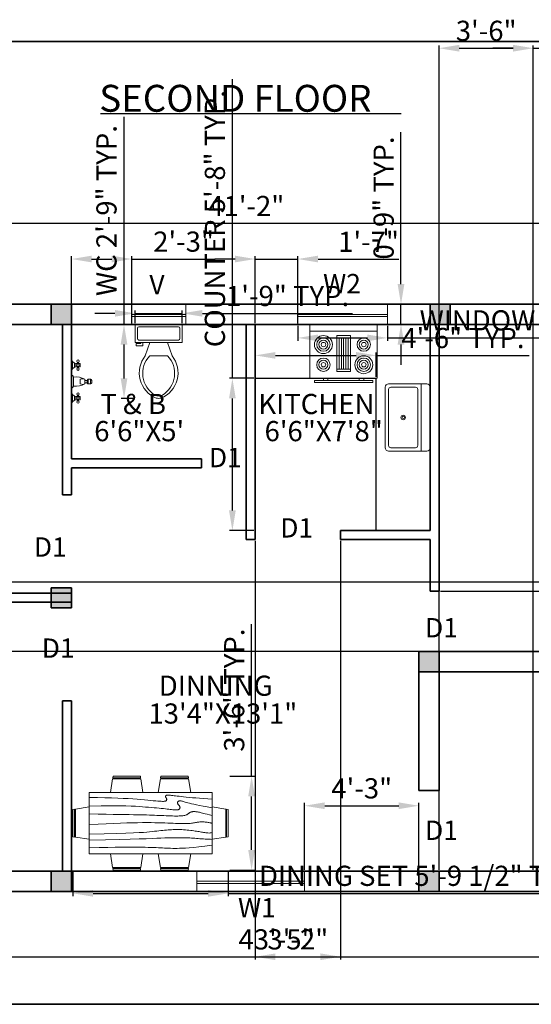
# Model space of a CAD drawing. Units: inches. Extents: x -281 to 2337, y 1647 to 2113.
# Tile 2 of 6: x 1230 to 1459, y 1674 to 2113. Entities that reach past the tile are written whole.
import ezdxf

# ---------------------------------------------------------------- set-up
doc = ezdxf.new("R2010")
doc.units = ezdxf.units.IN
for name, color, linetype, lineweight in [('A-ANNO-DIMS', 242, 'Continuous', 18), ('A-ANNO-IDEN', 11, 'Continuous', 18), ('A-ANNO-TEXT', 7, 'Continuous', 25), ('A-ANNO-TTLB', 7, 'Continuous', 35), ('A-AREA-IDEN', 7, 'Continuous', 18), ('A-COLS', 1, 'Continuous', 35), ('A-EQPM', 8, 'Continuous', 18), ('A-FLOR-CASE', 8, 'Continuous', 25), ('A-FLOR-FIXT', 8, 'Continuous', 18), ('A-FURN', 8, 'Continuous', 18), ('A-GLAZ', 3, 'Continuous', 18), ('A-WALL', 7, 'Continuous', 35)]:
    doc.layers.add(name, color=color, linetype=linetype, lineweight=lineweight)
doc.styles.get("Standard").update_dxf_attribs({"font": 'arial.ttf'})
doc.dimstyles.new('ISO-25', dxfattribs={"dimtxt": 9, "dimasz": 9, "dimexe": 1.25, "dimexo": 0.625, "dimgap": 2, "dimtad": 1, "dimdec": 1, "dimlunit": 4, "dimtxsty": 'Standard', "dimcen": 2.5, "dimadec": 0, "dimazin": 0, "dimtfac": 1, "dimtdec": 1, "dimtmove": 0, "dimatfit": 3, "dimfxl": 1, "dimarcsym": 0})

# ---------------------------------------------------------------- blocks, each defined once
blk = doc.blocks.new('Dining Set - 36 x 72 in.')
for p, q in [((-22.2343, 26.00059), (-23.4847, 17.99762)), ((-22.2304, 26), (-5.7608, 26)), ((-22, 27.5), (-22.1562, 26.50042)), ((-5.8416, 26.5), (-22.1534, 26.5)), ((-22, 27.5), (-6, 27.5)), ((-5.8437, 26.49966), (-6, 27.5)), ((-4.5152, 17.99762), (-5.7655, 25.99926)), ((5.7657, 26.00059), (4.5153, 17.99762)), ((5.7696, 26), (22.2392, 26)), ((6, 27.5), (5.8438, 26.50042)), ((22.1584, 26.5), (5.8466, 26.5)), ((6, 27.5), (22, 27.5)), ((22.1563, 26.49966), (22, 27.5)), ((23.4848, 17.99762), (22.2345, 25.99926)), ((36, 18), (-36, 18)), ((-36, 18), (-36, -18)), ((36, -18), (36, 18)), ((-45.5, 8), (-44.5004, 8.15617)), ((-45.5, 8), (-45.5, -8)), ((-44.5, -8.15843), (-44.5, 8.15338)), ((-44.0006, 8.23428), (-35.9976, 9.48474)), ((-44, 8.23041), (-44, -8.23915)), ((44.0006, 8.23428), (35.9976, 9.48474)), ((44, 8.23041), (44, -8.23915)), ((44.5, -8.15843), (44.5, 8.15338)), ((45.5, 8), (44.5005, 8.15617)), ((45.5, 8), (45.5, -8)), ((-44.4997, -8.15631), (-45.5, -8)), ((-35.9976, -9.48476), (-43.9993, -8.2345)), ((35.9976, -9.48476), (43.9993, -8.2345)), ((44.4997, -8.15631), (45.5, -8)), ((-36, -18), (36, -18)), ((-22.2343, -26.0006), (-23.4847, -17.99762)), ((-4.5152, -17.99762), (-5.7655, -25.99928)), ((5.7657, -26.0006), (4.5153, -17.99762)), ((23.4848, -17.99762), (22.2345, -25.99928)), ((-22.2304, -26), (-5.7608, -26)), ((-22, -27.5), (-22.1562, -26.50044)), ((-5.8416, -26.5), (-22.1534, -26.5)), ((-22, -27.5), (-6, -27.5)), ((-5.8437, -26.49967), (-6, -27.5)), ((5.7696, -26), (22.2392, -26)), ((6, -27.5), (5.8438, -26.50044)), ((22.1584, -26.5), (5.8466, -26.5)), ((6, -27.5), (22, -27.5)), ((22.1563, -26.49967), (22, -27.5))]:
    blk.add_line(p, q)
for points in [[(-36, 15), (-31.1772, 14.97754), (-26.8079, 14.91406), (-22.8538, 14.81543), (-19.276, 14.6875), (-16.0362, 14.53613), (-13.0957, 14.36718), (-10.4159, 14.18652), (-7.9583, 14), (-5.6904, 13.81315), (-3.6035, 13.63021), (-1.6954, 13.45508), (0.0365, 13.29166), (1.5945, 13.14388), (2.9811, 13.01562), (4.1988, 12.9108), (5.25, 12.83333), (6.1393, 12.78613), (6.8802, 12.76823), (7.4883, 12.77767), (7.9792, 12.8125), (8.3685, 12.87077), (8.6719, 12.95052), (8.9049, 13.0498), (9.0833, 13.16666), (9.2205, 13.29899), (9.3216, 13.44401), (9.3895, 13.59879), (9.4271, 13.76041), (9.4373, 13.92594), (9.4232, 14.09245), (9.3875, 14.257), (9.3333, 14.41666), (9.2638, 14.56917), (9.1836, 14.71484), (9.0975, 14.85465), (9.0104, 14.98958), (8.9272, 15.1206), (8.8529, 15.2487), (8.7922, 15.37483), (8.75, 15.5), (8.7305, 15.62467), (8.7344, 15.74739), (8.7617, 15.86621), (8.8125, 15.97916), (8.8867, 16.08431), (8.9844, 16.17968), (9.1055, 16.26334), (9.25, 16.33333), (9.4189, 16.38802), (9.6172, 16.42708), (9.8506, 16.45052), (10.125, 16.45833), (10.4463, 16.45052), (10.8203, 16.42708), (11.2529, 16.38802), (11.75, 16.33333), (12.3184, 16.26318), (12.9694, 16.17838), (13.7151, 16.07991), (14.5677, 15.96875), (15.5395, 15.84586), (16.6426, 15.71224), (17.8893, 15.56884), (19.2917, 15.41666), (20.859, 15.25667), (22.5879, 15.08984), (24.4721, 14.91715), (26.5052, 14.73958), (28.6809, 14.5581), (30.9929, 14.3737), (33.4347, 14.18733), (36, 14)], [(-36, 10), (-28.9766, 10.14274), (-23.1725, 10.20442), (-18.4241, 10.19775), (-14.5677, 10.13541), (-11.4399, 10.03011), (-8.877, 9.89453), (-6.7154, 9.74137), (-4.7917, 9.58333), (-2.9698, 9.43082), (-1.2246, 9.28515), (0.4415, 9.14534), (2.026, 9.01041), (3.5266, 8.87939), (4.9408, 8.7513), (6.266, 8.62516), (7.5, 8.5), (8.6411, 8.37549), (9.6914, 8.2539), (10.6538, 8.13818), (11.5312, 8.03125), (12.3267, 7.93603), (13.043, 7.85547), (13.6831, 7.79248), (14.25, 7.75), (14.7471, 7.7303), (15.1797, 7.73307), (15.5537, 7.75732), (15.875, 7.80208), (16.1494, 7.86637), (16.3828, 7.94922), (16.5811, 8.04964), (16.75, 8.16666), (16.8944, 8.29915), (17.0143, 8.44531), (17.1089, 8.60319), (17.1771, 8.77083), (17.218, 8.94629), (17.2305, 9.1276), (17.2137, 9.31282), (17.1667, 9.5), (17.0895, 9.6875), (16.987, 9.875), (16.8649, 10.0625), (16.7292, 10.25), (16.5856, 10.4375), (16.4401, 10.625), (16.2985, 10.8125), (16.1667, 11), (16.05, 11.18733), (15.9518, 11.3737), (15.8752, 11.5581), (15.8229, 11.73958), (15.798, 11.91715), (15.8034, 12.08984), (15.842, 12.25667), (15.9167, 12.41666), (16.0295, 12.56836), (16.1784, 12.70833), (16.3605, 12.83268), (16.5729, 12.9375), (16.8127, 13.01888), (17.0768, 13.07291), (17.3625, 13.0957), (17.6667, 13.08333), (17.9894, 13.03312), (18.3418, 12.94726), (18.7382, 12.82918), (19.1927, 12.68229), (19.7195, 12.51001), (20.3327, 12.31575), (21.0465, 12.10294), (21.875, 11.875), (22.8357, 11.63354), (23.959, 11.37304), (25.2786, 11.08618), (26.8282, 10.76562), (28.6414, 10.40405), (30.752, 9.99414), (33.1936, 9.52856), (36, 9)], [(-36, 5.5), (-30.7157, 5.3348), (-26.069, 5.20963), (-21.9946, 5.11767), (-18.4271, 5.05208), (-15.3009, 5.00602), (-12.5508, 4.97265), (-10.1112, 4.94515), (-7.9167, 4.91666), (-5.909, 4.88167), (-4.0586, 4.83984), (-2.3429, 4.79215), (-0.7396, 4.73958), (0.7739, 4.6831), (2.22, 4.6237), (3.6213, 4.56233), (5, 4.5), (6.373, 4.43782), (7.7344, 4.3776), (9.0723, 4.32129), (10.375, 4.27083), (11.6309, 4.22819), (12.8281, 4.19531), (13.9551, 4.17415), (15, 4.16666), (15.954, 4.17448), (16.819, 4.19791), (17.6001, 4.23698), (18.3021, 4.29166), (18.9299, 4.36198), (19.4883, 4.44791), (19.9823, 4.54948), (20.4167, 4.66666), (20.7969, 4.79899), (21.1302, 4.94401), (21.4245, 5.09879), (21.6875, 5.26041), (21.9271, 5.42594), (22.1511, 5.59245), (22.3672, 5.757), (22.5834, 5.91666), (22.8065, 6.06868), (23.0404, 6.21093), (23.2879, 6.34147), (23.5521, 6.45833), (23.8358, 6.55957), (24.142, 6.64323), (24.4735, 6.70735), (24.8334, 6.75), (25.2235, 6.76969), (25.642, 6.76692), (26.0858, 6.74267), (26.5521, 6.69791), (27.0379, 6.63362), (27.5404, 6.55078), (28.0565, 6.45036), (28.5834, 6.33333), (29.1242, 6.19987), (29.7071, 6.04687), (30.3661, 5.87044), (31.1354, 5.66666), (32.0493, 5.43164), (33.142, 5.16146), (34.4475, 4.85221), (36, 4.5)], [(-36, -1), (-30.7915, -0.6591), (-26.0195, -0.38216), (-21.6519, -0.16284), (-17.6563, 0.00521), (-14.0005, 0.12833), (-10.6523, 0.21289), (-7.5796, 0.26522), (-4.75, 0.29166), (-2.134, 0.29793), (0.2878, 0.28711), (2.5317, 0.26163), (4.6146, 0.22396), (6.5529, 0.17651), (8.3633, 0.12174), (10.0623, 0.06209), (11.6667, 0), (13.1899, -0.06201), (14.6341, -0.1211), (15.9982, -0.17432), (17.2813, -0.21875), (18.4823, -0.25147), (19.6003, -0.26953), (20.6343, -0.27002), (21.5834, -0.25), (22.4481, -0.20768), (23.2357, -0.14584), (23.9549, -0.06836), (24.6146, 0.02083), (25.2235, 0.11784), (25.7904, 0.21875), (26.3241, 0.31966), (26.8334, 0.41666), (27.3265, 0.50618), (27.8099, 0.58593), (28.2894, 0.65397), (28.7709, 0.70833), (29.2601, 0.74707), (29.763, 0.76823), (30.2855, 0.76985), (30.8334, 0.75), (31.4088, 0.70784), (31.9994, 0.64713), (32.589, 0.57275), (33.1615, 0.48958), (33.7008, 0.4025), (34.1908, 0.3164), (34.6153, 0.23616), (34.9584, 0.16666), (35.2099, 0.11165), (35.3848, 0.07031), (35.504, 0.04069), (35.5886, 0.02083), (35.6594, 0.00879), (35.7377, 0.0026), (35.8442, 0.00032), (36, 0)], [(-36, -6.5), (-27.1843, -6.31267), (-20.084, -6.1263), (-14.469, -5.9419), (-10.1094, -5.76042), (-6.7752, -5.58285), (-4.2363, -5.41016), (-2.2629, -5.24333), (-0.625, -5.08334), (0.8708, -4.93099), (2.2715, -4.78646), (3.5872, -4.64974), (4.8281, -4.52084), (6.0046, -4.39974), (7.127, -4.28646), (8.2053, -4.18099), (9.25, -4.08334), (10.2705, -3.99382), (11.2734, -3.91407), (12.2647, -3.84603), (13.25, -3.79167), (14.2354, -3.75293), (15.2266, -3.73177), (16.2295, -3.73015), (17.25, -3.75), (18.2912, -3.79248), (19.3451, -3.85547), (20.4009, -3.93604), (21.4479, -4.03125), (22.4754, -4.13819), (23.4727, -4.25391), (24.4289, -4.37549), (25.3334, -4.5), (26.1785, -4.62492), (26.9694, -4.74935), (27.7145, -4.87281), (28.4219, -4.99479), (29.1, -5.11483), (29.7572, -5.23242), (30.4016, -5.34709), (31.0417, -5.45834), (31.6837, -5.56437), (32.3262, -5.65821), (32.9658, -5.73153), (33.599, -5.77604), (34.2224, -5.78345), (34.8327, -5.74545), (35.4264, -5.65373), (36, -5.5)], [(-36, -10), (-26.4022, -9.81299), (-18.4675, -9.62891), (-11.9839, -9.45069), (-6.7396, -9.28125), (-2.5226, -9.12354), (0.8789, -8.98047), (3.6769, -8.85498), (6.0833, -8.75), (8.2767, -8.66765), (10.3021, -8.60677), (12.1712, -8.56543), (13.8958, -8.54167), (15.4876, -8.53353), (16.9583, -8.53907), (18.3197, -8.55632), (19.5834, -8.58334), (20.7616, -8.61841), (21.8685, -8.66081), (22.9188, -8.71004), (23.9271, -8.76563), (24.9081, -8.82707), (25.8763, -8.89388), (26.8465, -8.96558), (27.8334, -9.04167), (28.8474, -9.12118), (29.8828, -9.20117), (30.93, -9.27824), (31.9792, -9.34896), (33.0205, -9.40991), (34.0443, -9.45768), (35.0407, -9.48885), (36, -9.5)], [(-36, -14.5), (-30.0881, -14.33513), (-25.0332, -14.21224), (-20.7312, -14.12647), (-17.0781, -14.07292), (-13.97, -14.04671), (-11.3027, -14.04297), (-8.9724, -14.05681), (-6.875, -14.08334), (-4.9224, -14.11833), (-3.0905, -14.16016), (-1.3709, -14.20785), (0.2448, -14.26042), (1.7647, -14.3169), (3.1973, -14.3763), (4.5507, -14.43767), (5.8333, -14.5), (7.0554, -14.5621), (8.235, -14.62175), (9.3922, -14.67652), (10.5469, -14.72396), (11.7192, -14.76164), (12.929, -14.78711), (14.1965, -14.79794), (15.5417, -14.79167), (16.9933, -14.76424), (18.6152, -14.70508), (20.4804, -14.60197), (22.6615, -14.44271), (25.2312, -14.21509), (28.2624, -13.9069), (31.8277, -13.50594), (36, -13)]]:
    blk.add_lwpolyline(points)
blk = doc.blocks.new('Toilet - top')
for p, q in [((9.5, -6), (9.5, -2)), ((-10, -8.5), (-8, -8.5)), ((-10, -9.5), (-10, -8.5)), ((-8, -8.5), (-8, -8)), ((-7, -8), (-7, -9.5)), ((-4, -8), (-6, -14)), ((4, -8), (6, -14)), ((-7, -9.5), (-10, -9.5)), ((4, -14), (-4, -14))]:
    blk.add_line(p, q)
blk.add_lwpolyline([(10.5, -8), (10.5, 0), (-10.5, 0), (-10.5, -8)], close=True)
for points in [[(-9.5, -2), (-9.5, -6)], [(8.5, -1), (-8.5, -1)], [(-8.5, -7), (8.5, -7)]]:
    blk.add_lwpolyline(points)
for centre, radius, start, end in [((-8.62, -1.88), 0.884, 81.8699, 188.1301), ((8.62, -1.88), 0.884, 351.8699, 98.1301), ((-8.62, -6.12), 0.884, 171.8699, 278.1301), ((8.62, -6.12), 0.884, 261.8699, 8.1301), ((3.52, -21.58), 12.17, 141.4691, 247.9714), ((4.2, -21.82), 11.33, 136.3677, 238.9468), ((-3.52, -21.58), 12.17, 292.0284, 38.5307), ((-4.2, -21.82), 11.33, 301.053, 43.6321), ((0, -27.88), 4, 245.7318, 294.2682), ((0, -29), 4, 254.8605, 285.1395)]:
    blk.add_arc(centre, radius, start, end)
blk = doc.blocks.new('Faucet - Bathroom front')
for p, q in [((-0.5, 4.25), (0.5, 4.25)), ((0.5, 3.75), (-0.5, 3.75)), ((-0.5, 3), (0.5, 3)), ((-0.25, 3), (-0.25, 3.5)), ((0.25, 3.5), (0.25, 3)), ((-5, 0), (-2.25, 0)), ((-4.5087, 0.25), (-2.7408, 0.25)), ((-4, 1.625), (-4.25, 1.625)), ((-4, 1.375), (-4.25, 1.375)), ((-3.1442, 0.75), (-4.0979, 0.75)), ((-3.25, 1.625), (-3, 1.625)), ((-3.25, 1.375), (-3, 1.375)), ((-1.5, 0), (1.5, 0)), ((-1, 0.5), (1, 0.5)), ((0.5, 2), (-0.5, 2)), ((2.25, 0), (5, 0)), ((2.7413, 0.25), (4.5092, 0.25)), ((3.25, 1.625), (3, 1.625)), ((3.25, 1.375), (3, 1.375)), ((4.1058, 0.75), (3.1521, 0.75)), ((4, 1.625), (4.25, 1.625)), ((4, 1.375), (4.25, 1.375))]:
    blk.add_line(p, q)
for points in [[(-0.25, 4.5), (0.25, 4.5)], [(-0.5, 3.75), (-0.5, 4.25)], [(0.25, 3.5), (-0.25, 3.5)], [(0.5, 4.25), (0.5, 3.75)]]:
    blk.add_lwpolyline(points)
for points in [[(-4, 1), (-4, 2), (-3.25, 2), (-3.25, 1)], [(3.25, 1), (3.25, 2), (4, 2), (4, 1)]]:
    blk.add_lwpolyline(points, close=True)
for centre in [(-4.5, 1.5), (-3.625, 1.5), (-2.75, 1.5), (2.75, 1.5), (3.625, 1.5), (4.5, 1.5)]:
    blk.add_circle(centre, 0.2795)
for centre, radius, start, end in [((-0.2575, 4.2575), 0.2426, 88.22243, 181.7776), ((0.2575, 4.2575), 0.2426, 358.2224, 91.77757), ((3, 1), 4.0311, 150.2551, 187.125), ((0.6413, 2.5), 1.246, 156.3417, 203.6583), ((-0.2575, 3.7425), 0.2426, 178.2224, 271.7776), ((0.2575, 3.7425), 0.2426, 268.2224, 1.777565), ((-3, 1), 4.0311, 352.875, 29.74488), ((-0.6413, 2.5), 1.246, 336.3417, 23.65835), ((-5.375, 1.375), 1.4252, 285.2551, 344.7449), ((-1.875, 1.375), 1.4252, 195.2551, 254.7449), ((-0.7962, -0.2038), 0.7327, 106.1502, 163.8498), ((0.7962, -0.2038), 0.7327, 16.1502, 73.84979), ((1.875, 1.375), 1.4252, 285.2551, 344.7449), ((5.375, 1.375), 1.4252, 195.2551, 254.7449)]:
    blk.add_arc(centre, radius, start, end)
blk = doc.blocks.new('Range-Oven - 30 in top')
for p, q in [((0, -3), (30, -3)), ((12, -6), (18, -6)), ((13, -20), (13, -6)), ((14, -6), (14, -20)), ((15, -20), (15, -6)), ((16, -6), (16, -20)), ((17, -20), (17, -6)), ((18, -20), (12, -20)), ((6, -24), (6, -25)), ((8, -25), (8, -24)), ((22, -25), (22, -24)), ((24, -24), (24, -25))]:
    blk.add_line(p, q)
for points in [[(0, -24), (0, 0), (30, 0), (30, -24)], [(12, -21), (12, -5), (18, -5), (18, -21)], [(2, -26), (2, -25), (28, -25), (28, -26)]]:
    blk.add_lwpolyline(points, close=True)
for centre, radius in [((6, -9), 4), ((6, -9), 3), ((6, -9), 2), ((6, -9), 1), ((24, -9), 3), ((24, -9), 2), ((24, -9), 1), ((6, -18), 3), ((6, -18), 2), ((6, -18), 1), ((24, -18), 4), ((24, -18), 3), ((24, -18), 2), ((24, -18), 1)]:
    blk.add_circle(centre, radius)
blk = doc.blocks.new('Sink-single - 30 in top')
blk.add_line((-15, -3.999996), (15, -3.999996))
for points in [[(-13.5, 0), (13.5, 0)], [(-15, -18.499996), (-15, -1.5)], [(15, -1.5), (15, -18.499996)], [(-13.5, -17.499996), (-13.5, -6.499996)], [(-12.5, -5.499996), (12.5, -5.499996)], [(13.5, -6.499996), (13.5, -17.499996)], [(13.5, -19.999996), (-13.5, -19.999996)], [(12.5, -18.499996), (-12.5, -18.499996)]]:
    blk.add_lwpolyline(points)
for radius in [1, 0.5]:
    blk.add_circle((0, -11.999996), radius)
for centre, radius, start, end in [((-13.5, -1.5), 1.5, 90, 180), ((13.5, -1.5), 1.5, 0, 90), ((-12.5, -6.499996), 1, 90, 180), ((12.5, -6.499996), 1, 0, 90), ((-12.5, -17.499996), 1, 180, 270), ((12.5, -17.499996), 1, 270, 0), ((-13.5, -18.499996), 1.5, 180, 270), ((13.5, -18.499996), 1.5, 270, 0)]:
    blk.add_arc(centre, radius, start, end)
blk = doc.blocks.new('*D8')
at = {"layer": 'A-ANNO-DIMS', "color": 0, "lineweight": -2, "transparency": 16777216}
for p, q in [((1084.42, 1986.77), (1084.42, 2023.6)), ((1093.42, 2022.35), (1569.42, 2022.35)), ((1578.42, 1986.77), (1578.42, 2023.6))]:
    blk.add_line(p, q, dxfattribs=at)
at = {"layer": 'A-ANNO-DIMS', "color": 0, "transparency": 16777216}
for points in [[(1093.42, 2023.85), (1093.42, 2020.85), (1084.42, 2022.35)], [(1569.42, 2023.85), (1569.42, 2020.85), (1578.42, 2022.35)]]:
    blk.add_solid(points, dxfattribs=at)
at = {"layer": 'Defpoints', "color": 0, "transparency": 16777216}
for p in [(1578.42, 2022.35), (1084.42, 1986.15), (1578.42, 1986.15)]:
    blk.add_point(p, dxfattribs=at)
at = {"layer": 'A-ANNO-DIMS', "color": 0, "transparency": 16777216, "insert": (1331.42, 2028.86), "char_height": 9, "attachment_point": 5}
blk.add_mtext('41\'-2"', dxfattribs=at)
blk = doc.blocks.new('COL-9x9')
h = blk.add_hatch(color=256)
h.dxf.hatch_style = 1
h.paths.add_polyline_path([(9, 9), (0, 9), (0, 0), (9, 0)])
for p, q in [((0, 9), (9, 9)), ((0, 0), (0, 9)), ((9, 9), (9, 0)), ((9, 0), (0, 0))]:
    blk.add_line(p, q)
blk = doc.blocks.new('WIN-W1-48')
for p, q in [((0, 48), (9, 48)), ((3.5, 0), (3.5, 48)), ((4.5, 0), (4.5, 48)), ((0, 0), (9, 0))]:
    blk.add_line(p, q)
blk = doc.blocks.new('WIN-W2-40')
for p, q in [((0, 0), (0, 9)), ((40, 0), (40, 9)), ((0, 4.5), (40, 4.5)), ((0, 3.5), (40, 3.5))]:
    blk.add_line(p, q)
blk = doc.blocks.new('VENT-24')
for p, q in [((0, 0), (0, 9)), ((24, 0), (24, 9)), ((0, 4.5), (24, 4.5)), ((0, 3.5), (24, 3.5))]:
    blk.add_line(p, q)
blk = doc.blocks.new('COUNTER-L')
for p in [(0, 68), (54, 0)]:
    blk.add_line(p, (54, 68))
blk = doc.blocks.new('*D21')
at = {"layer": 'A-ANNO-DIMS', "color": 0, "lineweight": -2, "transparency": 16777216}
for p, q in [((1354.42, 1976.52), (1354.42, 1969.9)), ((1394.42, 1976.52), (1394.42, 1969.9)), ((1363.42, 1971.15), (1385.42, 1971.15)), ((1394.42, 1971.15), (1543.66, 1971.15))]:
    blk.add_line(p, q, dxfattribs=at)
at = {"layer": 'A-ANNO-DIMS', "color": 0, "transparency": 16777216}
for points in [[(1363.42, 1972.65), (1363.42, 1969.65), (1354.42, 1971.15)], [(1385.42, 1972.65), (1385.42, 1969.65), (1394.42, 1971.15)]]:
    blk.add_solid(points, dxfattribs=at)
at = {"layer": 'Defpoints', "color": 0, "transparency": 16777216}
for p in [(1354.42, 1977.15), (1394.42, 1977.15), (1394.42, 1971.15)]:
    blk.add_point(p, dxfattribs=at)
at = {"layer": 'A-ANNO-DIMS', "color": 0, "transparency": 16777216, "insert": (1473.54, 1977.81), "char_height": 9, "attachment_point": 5}
blk.add_mtext('WINDOW W2 3\'-4" TYP.', dxfattribs=at)
blk = doc.blocks.new('*D22')
at = {"layer": 'A-ANNO-DIMS', "color": 0, "lineweight": -2, "transparency": 16777216}
for p, q in [((1400.42, 1995.15), (1400.42, 2063.01)), ((1395.05, 1986.15), (1401.67, 1986.15)), ((1400.42, 1977.15), (1400.42, 1986.15)), ((1395.05, 1977.15), (1401.67, 1977.15)), ((1400.42, 1968.15), (1400.42, 1959.15))]:
    blk.add_line(p, q, dxfattribs=at)
at = {"layer": 'A-ANNO-DIMS', "color": 0, "transparency": 16777216}
for points in [[(1398.92, 1995.15), (1401.92, 1995.15), (1400.42, 1986.15)], [(1398.92, 1968.15), (1401.92, 1968.15), (1400.42, 1977.15)]]:
    blk.add_solid(points, dxfattribs=at)
at = {"layer": 'Defpoints', "color": 0, "transparency": 16777216}
for p in [(1394.42, 1986.15), (1400.42, 1986.15), (1394.42, 1977.15)]:
    blk.add_point(p, dxfattribs=at)
at = {"layer": 'A-ANNO-DIMS', "color": 0, "transparency": 16777216, "insert": (1393.83, 2033.58), "char_height": 9, "attachment_point": 5, "rotation": 90}
blk.add_mtext('0\'-9" TYP.', dxfattribs=at)
blk = doc.blocks.new('*D29')
at = {"layer": 'A-ANNO-DIMS', "color": 0, "lineweight": -2, "transparency": 16777216}
for p, q in [((1254.1, 1733.03), (1254.1, 1722.01)), ((1323.39, 1733.03), (1323.39, 1722.01)), ((1263.1, 1723.26), (1314.39, 1723.26)), ((1323.39, 1723.26), (1487.21, 1723.26))]:
    blk.add_line(p, q, dxfattribs=at)
at = {"layer": 'A-ANNO-DIMS', "color": 0, "transparency": 16777216}
for points in [[(1263.1, 1724.76), (1263.1, 1721.76), (1254.1, 1723.26)], [(1314.39, 1724.76), (1314.39, 1721.76), (1323.39, 1723.26)]]:
    blk.add_solid(points, dxfattribs=at)
at = {"layer": 'Defpoints', "color": 0, "transparency": 16777216}
for p in [(1254.1, 1733.65), (1323.39, 1733.65), (1323.39, 1723.26)]:
    blk.add_point(p, dxfattribs=at)
at = {"layer": 'A-ANNO-DIMS', "color": 0, "transparency": 16777216, "insert": (1409.8, 1729.91), "char_height": 9, "attachment_point": 5}
blk.add_mtext('DINING SET 5\'-9 1/2" TYP.', dxfattribs=at)
blk = doc.blocks.new('*D30')
at = {"layer": 'A-ANNO-DIMS', "color": 0, "lineweight": -2, "transparency": 16777216}
for p, q in [((1333.78, 1775.53), (1333.78, 1843.38)), ((1324.01, 1775.53), (1335.03, 1775.53)), ((1333.78, 1742.65), (1333.78, 1766.53)), ((1324.01, 1733.65), (1335.03, 1733.65))]:
    blk.add_line(p, q, dxfattribs=at)
at = {"layer": 'A-ANNO-DIMS', "color": 0, "transparency": 16777216}
for points in [[(1332.28, 1766.53), (1335.28, 1766.53), (1333.78, 1775.53)], [(1332.28, 1742.65), (1335.28, 1742.65), (1333.78, 1733.65)]]:
    blk.add_solid(points, dxfattribs=at)
at = {"layer": 'Defpoints', "color": 0, "transparency": 16777216}
for p in [(1323.39, 1775.53), (1333.78, 1775.53), (1323.39, 1733.65)]:
    blk.add_point(p, dxfattribs=at)
at = {"layer": 'A-ANNO-DIMS', "color": 0, "transparency": 16777216, "insert": (1327.18, 1813.95), "char_height": 9, "attachment_point": 5, "rotation": 90}
blk.add_mtext('3\'-6" TYP.', dxfattribs=at)
blk = doc.blocks.new('*D35')
at = {"layer": 'A-ANNO-DIMS', "color": 0, "lineweight": -2, "transparency": 16777216}
for p, q in [((1325.22, 1953.15), (1325.22, 2086.56)), ((1334.8, 1953.15), (1323.97, 1953.15)), ((1325.22, 1894.15), (1325.22, 1944.15)), ((1334.8, 1885.15), (1323.97, 1885.15))]:
    blk.add_line(p, q, dxfattribs=at)
at = {"layer": 'A-ANNO-DIMS', "color": 0, "transparency": 16777216}
for points in [[(1323.72, 1944.15), (1326.72, 1944.15), (1325.22, 1953.15)], [(1323.72, 1894.15), (1326.72, 1894.15), (1325.22, 1885.15)]]:
    blk.add_solid(points, dxfattribs=at)
at = {"layer": 'Defpoints', "color": 0, "transparency": 16777216}
for p in [(1325.22, 1953.15), (1335.42, 1953.15), (1335.42, 1885.15)]:
    blk.add_point(p, dxfattribs=at)
at = {"layer": 'A-ANNO-DIMS', "color": 0, "transparency": 16777216, "insert": (1318.57, 2024.36), "char_height": 9, "attachment_point": 5, "rotation": 90}
blk.add_mtext('COUNTER 5\'-8" TYP.', dxfattribs=at)
blk = doc.blocks.new('*D36')
at = {"layer": 'A-ANNO-DIMS', "color": 0, "lineweight": -2, "transparency": 16777216}
for p, q in [((1335.42, 1953.77), (1335.42, 1964.6)), ((1389.42, 1953.77), (1389.42, 1964.6)), ((1344.42, 1963.35), (1380.42, 1963.35)), ((1389.42, 1963.35), (1457.65, 1963.35))]:
    blk.add_line(p, q, dxfattribs=at)
at = {"layer": 'A-ANNO-DIMS', "color": 0, "transparency": 16777216}
for points in [[(1344.42, 1964.85), (1344.42, 1961.85), (1335.42, 1963.35)], [(1380.42, 1964.85), (1380.42, 1961.85), (1389.42, 1963.35)]]:
    blk.add_solid(points, dxfattribs=at)
at = {"layer": 'Defpoints', "color": 0, "transparency": 16777216}
for p in [(1389.42, 1963.35), (1335.42, 1953.15), (1389.42, 1953.15)]:
    blk.add_point(p, dxfattribs=at)
at = {"layer": 'A-ANNO-DIMS', "color": 0, "transparency": 16777216, "insert": (1428.04, 1969.94), "char_height": 9, "attachment_point": 5}
blk.add_mtext('4\'-6" TYP.', dxfattribs=at)
blk = doc.blocks.new('*D37')
at = {"layer": 'A-ANNO-DIMS', "color": 0, "lineweight": -2, "transparency": 16777216}
for p, q in [((1276.88, 1977.15), (1276.88, 2069.82)), ((1281.22, 1977.15), (1275.63, 1977.15)), ((1276.88, 1953.1), (1276.88, 1968.15)), ((1281.22, 1944.1), (1275.63, 1944.1))]:
    blk.add_line(p, q, dxfattribs=at)
at = {"layer": 'A-ANNO-DIMS', "color": 0, "transparency": 16777216}
for points in [[(1275.38, 1968.15), (1278.38, 1968.15), (1276.88, 1977.15)], [(1275.38, 1953.1), (1278.38, 1953.1), (1276.88, 1944.1)]]:
    blk.add_solid(points, dxfattribs=at)
at = {"layer": 'Defpoints', "color": 0, "transparency": 16777216}
for p in [(1276.88, 1977.15), (1281.84, 1977.15), (1281.84, 1944.1)]:
    blk.add_point(p, dxfattribs=at)
at = {"layer": 'A-ANNO-DIMS', "color": 0, "transparency": 16777216, "insert": (1270.23, 2027.98), "char_height": 9, "attachment_point": 5, "rotation": 90}
blk.add_mtext('WC 2\'-9" TYP.', dxfattribs=at)
blk = doc.blocks.new('*D38')
at = {"layer": 'A-ANNO-DIMS', "color": 0, "lineweight": -2, "transparency": 16777216}
for p, q in [((1272.84, 1982.11), (1263.84, 1982.11)), ((1281.84, 1977.77), (1281.84, 1983.36)), ((1281.84, 1982.11), (1302.84, 1982.11)), ((1302.84, 1977.77), (1302.84, 1983.36)), ((1311.84, 1982.11), (1378.85, 1982.11))]:
    blk.add_line(p, q, dxfattribs=at)
at = {"layer": 'A-ANNO-DIMS', "color": 0, "transparency": 16777216}
for points in [[(1272.84, 1983.61), (1272.84, 1980.61), (1281.84, 1982.11)], [(1311.84, 1983.61), (1311.84, 1980.61), (1302.84, 1982.11)]]:
    blk.add_solid(points, dxfattribs=at)
at = {"layer": 'Defpoints', "color": 0, "transparency": 16777216}
for p in [(1302.84, 1982.11), (1281.84, 1977.15), (1302.84, 1977.15)]:
    blk.add_point(p, dxfattribs=at)
at = {"layer": 'A-ANNO-DIMS', "color": 0, "transparency": 16777216, "insert": (1349.85, 1988.7), "char_height": 9, "attachment_point": 5}
blk.add_mtext('1\'-9" TYP.', dxfattribs=at)
blk = doc.blocks.new('*D42')
at = {"layer": 'A-ANNO-DIMS', "color": 0, "lineweight": -2, "transparency": 16777216}
for p, q in [((1084.42, 1723.52), (1084.42, 1693.7)), ((1605.42, 1723.52), (1605.42, 1693.7)), ((1093.42, 1694.95), (1596.42, 1694.95))]:
    blk.add_line(p, q, dxfattribs=at)
at = {"layer": 'A-ANNO-DIMS', "color": 0, "transparency": 16777216}
for points in [[(1093.42, 1696.45), (1093.42, 1693.45), (1084.42, 1694.95)], [(1596.42, 1696.45), (1596.42, 1693.45), (1605.42, 1694.95)]]:
    blk.add_solid(points, dxfattribs=at)
at = {"layer": 'Defpoints', "color": 0, "transparency": 16777216}
for p in [(1084.42, 1724.15), (1605.42, 1724.15), (1605.42, 1694.95)]:
    blk.add_point(p, dxfattribs=at)
at = {"layer": 'A-ANNO-DIMS', "color": 0, "transparency": 16777216, "insert": (1344.92, 1701.55), "char_height": 9, "attachment_point": 5}
blk.add_mtext('43\'-5"', dxfattribs=at)
blk = doc.blocks.new('*D57')
at = {"layer": 'A-ANNO-DIMS', "color": 0, "lineweight": -2, "transparency": 16777216}
for p, q in [((1577.8, 1862.15), (1053.97, 1862.15)), ((1055.22, 1840.15), (1055.22, 1853.15)), ((1577.8, 1831.15), (1053.97, 1831.15))]:
    blk.add_line(p, q, dxfattribs=at)
at = {"layer": 'A-ANNO-DIMS', "color": 0, "transparency": 16777216}
for points in [[(1053.72, 1853.15), (1056.72, 1853.15), (1055.22, 1862.15)], [(1053.72, 1840.15), (1056.72, 1840.15), (1055.22, 1831.15)]]:
    blk.add_solid(points, dxfattribs=at)
at = {"layer": 'Defpoints', "color": 0, "transparency": 16777216}
for p in [(1055.22, 1862.15), (1578.42, 1862.15), (1578.42, 1831.15)]:
    blk.add_point(p, dxfattribs=at)
at = {"layer": 'A-ANNO-DIMS', "color": 0, "transparency": 16777216, "insert": (1048.71, 1846.65), "char_height": 9, "attachment_point": 5, "rotation": 90}
blk.add_mtext('2\'-7"', dxfattribs=at)
blk = doc.blocks.new('*D58')
at = {"layer": 'A-ANNO-DIMS', "color": 0, "lineweight": -2, "transparency": 16777216}
for p, q in [((1634.62, 1858.15), (1634.62, 1895.23)), ((1418.05, 1858.15), (1635.87, 1858.15)), ((1634.62, 1840.15), (1634.62, 1849.15)), ((1418.05, 1831.15), (1635.87, 1831.15))]:
    blk.add_line(p, q, dxfattribs=at)
at = {"layer": 'A-ANNO-DIMS', "color": 0, "transparency": 16777216}
for points in [[(1633.12, 1849.15), (1636.12, 1849.15), (1634.62, 1858.15)], [(1633.12, 1840.15), (1636.12, 1840.15), (1634.62, 1831.15)]]:
    blk.add_solid(points, dxfattribs=at)
at = {"layer": 'Defpoints', "color": 0, "transparency": 16777216}
for p in [(1417.42, 1858.15), (1634.62, 1858.15), (1417.42, 1831.15)]:
    blk.add_point(p, dxfattribs=at)
at = {"layer": 'A-ANNO-DIMS', "color": 0, "transparency": 16777216, "insert": (1628.03, 1881.19), "char_height": 9, "attachment_point": 5, "rotation": 90}
blk.add_mtext('2\'-3"', dxfattribs=at)
blk = doc.blocks.new('*D60')
at = {"layer": 'A-ANNO-DIMS', "color": 0, "lineweight": -2, "transparency": 16777216}
for p, q in [((1417.42, 1733.77), (1417.42, 2101.68)), ((1459.42, 1733.77), (1459.42, 2101.68)), ((1426.42, 2100.43), (1450.42, 2100.43))]:
    blk.add_line(p, q, dxfattribs=at)
at = {"layer": 'A-ANNO-DIMS', "color": 0, "transparency": 16777216}
for points in [[(1426.42, 2101.93), (1426.42, 2098.93), (1417.42, 2100.43)], [(1450.42, 2101.93), (1450.42, 2098.93), (1459.42, 2100.43)]]:
    blk.add_solid(points, dxfattribs=at)
at = {"layer": 'Defpoints', "color": 0, "transparency": 16777216}
for p in [(1459.42, 2100.43), (1417.42, 1733.15), (1459.42, 1733.15)]:
    blk.add_point(p, dxfattribs=at)
at = {"layer": 'A-ANNO-DIMS', "color": 0, "transparency": 16777216, "insert": (1438.42, 2107.03), "char_height": 9, "attachment_point": 5}
blk.add_mtext('3\'-6"', dxfattribs=at)
blk = doc.blocks.new('*D61')
at = {"layer": 'A-ANNO-DIMS', "color": 0, "lineweight": -2, "transparency": 16777216}
for p, q in [((1459.42, 1822.77), (1459.42, 2101.68)), ((1469.42, 1822.77), (1469.42, 2101.68)), ((1450.42, 2100.43), (1441.42, 2100.43)), ((1459.42, 2100.43), (1469.42, 2100.43)), ((1478.42, 2100.43), (1522.34, 2100.43))]:
    blk.add_line(p, q, dxfattribs=at)
at = {"layer": 'A-ANNO-DIMS', "color": 0, "transparency": 16777216}
for points in [[(1450.42, 2101.93), (1450.42, 2098.93), (1459.42, 2100.43)], [(1478.42, 2101.93), (1478.42, 2098.93), (1469.42, 2100.43)]]:
    blk.add_solid(points, dxfattribs=at)
at = {"layer": 'Defpoints', "color": 0, "transparency": 16777216}
for p in [(1469.42, 2100.43), (1459.42, 1822.15), (1469.42, 1822.15)]:
    blk.add_point(p, dxfattribs=at)
at = {"layer": 'A-ANNO-DIMS', "color": 0, "transparency": 16777216, "insert": (1504.88, 2107.03), "char_height": 9, "attachment_point": 5}
blk.add_mtext('0\'-10"', dxfattribs=at)
blk = doc.blocks.new('*D62')
at = {"layer": 'A-ANNO-DIMS', "color": 0, "lineweight": -2, "transparency": 16777216}
for p, q in [((1335.42, 1880.52), (1335.42, 1693.7)), ((1373.42, 1880.52), (1373.42, 1693.7)), ((1344.42, 1694.95), (1364.42, 1694.95))]:
    blk.add_line(p, q, dxfattribs=at)
at = {"layer": 'A-ANNO-DIMS', "color": 0, "transparency": 16777216}
for points in [[(1344.42, 1696.45), (1344.42, 1693.45), (1335.42, 1694.95)], [(1364.42, 1696.45), (1364.42, 1693.45), (1373.42, 1694.95)]]:
    blk.add_solid(points, dxfattribs=at)
at = {"layer": 'Defpoints', "color": 0, "transparency": 16777216}
for p in [(1335.42, 1881.15), (1373.42, 1881.15), (1373.42, 1694.95)]:
    blk.add_point(p, dxfattribs=at)
at = {"layer": 'A-ANNO-DIMS', "color": 0, "transparency": 16777216, "insert": (1354.42, 1701.55), "char_height": 9, "attachment_point": 5}
blk.add_mtext('3\'-2"', dxfattribs=at)
blk = doc.blocks.new('*D64')
at = {"layer": 'A-ANNO-DIMS', "color": 0, "lineweight": -2, "transparency": 16777216}
for p, q in [((1253.42, 1977.77), (1253.42, 2007.6)), ((1262.42, 2006.35), (1271.42, 2006.35)), ((1280.42, 1977.77), (1280.42, 2007.6)), ((1280.42, 2006.35), (1317.5, 2006.35))]:
    blk.add_line(p, q, dxfattribs=at)
at = {"layer": 'A-ANNO-DIMS', "color": 0, "transparency": 16777216}
for points in [[(1262.42, 2007.85), (1262.42, 2004.85), (1253.42, 2006.35)], [(1271.42, 2007.85), (1271.42, 2004.85), (1280.42, 2006.35)]]:
    blk.add_solid(points, dxfattribs=at)
at = {"layer": 'Defpoints', "color": 0, "transparency": 16777216}
for p in [(1280.42, 2006.35), (1253.42, 1977.15), (1280.42, 1977.15)]:
    blk.add_point(p, dxfattribs=at)
at = {"layer": 'A-ANNO-DIMS', "color": 0, "transparency": 16777216, "insert": (1303.46, 2012.95), "char_height": 9, "attachment_point": 5}
blk.add_mtext('2\'-3"', dxfattribs=at)
blk = doc.blocks.new('*D66')
at = {"layer": 'A-ANNO-DIMS', "color": 0, "lineweight": -2, "transparency": 16777216}
for p, q in [((1357.42, 1733.77), (1357.42, 1763.6)), ((1366.42, 1762.35), (1399.42, 1762.35)), ((1408.42, 1733.77), (1408.42, 1763.6))]:
    blk.add_line(p, q, dxfattribs=at)
at = {"layer": 'A-ANNO-DIMS', "color": 0, "transparency": 16777216}
for points in [[(1366.42, 1763.85), (1366.42, 1760.85), (1357.42, 1762.35)], [(1399.42, 1763.85), (1399.42, 1760.85), (1408.42, 1762.35)]]:
    blk.add_solid(points, dxfattribs=at)
at = {"layer": 'Defpoints', "color": 0, "transparency": 16777216}
for p in [(1408.42, 1762.35), (1357.42, 1733.15), (1408.42, 1733.15)]:
    blk.add_point(p, dxfattribs=at)
at = {"layer": 'A-ANNO-DIMS', "color": 0, "transparency": 16777216, "insert": (1382.92, 1768.95), "char_height": 9, "attachment_point": 5}
blk.add_mtext('4\'-3"', dxfattribs=at)
blk = doc.blocks.new('*D68')
at = {"layer": 'A-ANNO-DIMS', "color": 0, "lineweight": -2, "transparency": 16777216}
for p, q in [((1326.42, 2006.35), (1317.42, 2006.35)), ((1335.42, 1977.77), (1335.42, 2007.6)), ((1335.42, 2006.35), (1354.42, 2006.35)), ((1354.42, 1977.77), (1354.42, 2007.6)), ((1363.42, 2006.35), (1399.5, 2006.35))]:
    blk.add_line(p, q, dxfattribs=at)
at = {"layer": 'A-ANNO-DIMS', "color": 0, "transparency": 16777216}
for points in [[(1326.42, 2007.85), (1326.42, 2004.85), (1335.42, 2006.35)], [(1363.42, 2007.85), (1363.42, 2004.85), (1354.42, 2006.35)]]:
    blk.add_solid(points, dxfattribs=at)
at = {"layer": 'Defpoints', "color": 0, "transparency": 16777216}
for p in [(1354.42, 2006.35), (1335.42, 1977.15), (1354.42, 1977.15)]:
    blk.add_point(p, dxfattribs=at)
at = {"layer": 'A-ANNO-DIMS', "color": 0, "transparency": 16777216, "insert": (1385.96, 2012.87), "char_height": 9, "attachment_point": 5}
blk.add_mtext('1\'-7"', dxfattribs=at)

msp = doc.modelspace()

# ---------------------------------------------------------------- linework, layer by layer
at = {"layer": 'A-ANNO-TEXT'}
msp.add_line((1266.46, 2071.23), (1400.51, 2071.23), dxfattribs=at)
at = {"layer": 'A-ANNO-TTLB'}
msp.add_lwpolyline([(1037.79, 2103.48), (2323.1, 2103.48), (2323.1, 1673.73), (1037.79, 1673.73)], close=True, dxfattribs=at)
at = {"layer": 'A-GLAZ'}
msp.add_line((1357.42, 1733.15), (1357.42, 1724.15), dxfattribs=at)
at = {"layer": 'A-WALL'}
for p, q in [((1084.42, 1986.15), (1605.42, 1986.15)), ((1253.42, 1917.15), (1253.42, 1986.15)), ((1413.42, 1986.15), (1413.42, 1885.15)), ((1093.42, 1977.15), (1601.42, 1977.15)), ((1249.42, 1977.15), (1249.42, 1901.15)), ((1249.42, 1901.15), (1249.42, 1977.15)), ((1253.42, 1977.15), (1253.42, 1917.15)), ((1331.42, 1977.15), (1331.42, 1881.15)), ((1335.42, 1977.15), (1335.42, 1881.15)), ((1417.42, 1977.15), (1417.42, 1858.15)), ((1253.42, 1917.15), (1311.42, 1917.15)), ((1311.42, 1917.15), (1311.42, 1913.15)), ((1253.42, 1913.15), (1311.42, 1913.15)), ((1253.42, 1901.15), (1253.42, 1913.15)), ((1253.42, 1913.15), (1253.42, 1901.15)), ((1253.42, 1901.15), (1249.42, 1901.15)), ((1331.42, 1881.15), (1335.42, 1881.15)), ((1373.42, 1885.15), (1373.42, 1881.15)), ((1373.42, 1885.15), (1413.42, 1885.15)), ((1373.42, 1881.15), (1413.42, 1881.15)), ((1413.42, 1881.15), (1413.42, 1858.15)), ((1253.42, 1857.15), (1084.42, 1857.15)), ((1253.42, 1857.15), (1253.42, 1853.15)), ((1413.42, 1858.15), (1417.42, 1858.15)), ((1253.42, 1853.15), (1093.42, 1853.15)), ((1408.42, 1831.15), (1605.42, 1831.15)), ((1408.42, 1831.15), (1408.42, 1769.15)), ((1417.42, 1822.15), (1605.42, 1822.15)), ((1417.42, 1822.15), (1417.42, 1769.15)), ((1249.42, 1733.15), (1249.42, 1809.15)), ((1253.42, 1809.15), (1249.42, 1809.15)), ((1253.42, 1724.15), (1253.42, 1809.15)), ((1408.42, 1769.15), (1417.42, 1769.15)), ((1249.42, 1733.15), (1093.42, 1733.15)), ((1413.42, 1733.15), (1253.42, 1733.15)), ((1408.42, 1733.15), (1408.42, 1724.15)), ((1605.42, 1733.15), (1413.42, 1733.15)), ((1417.42, 1733.15), (1417.42, 1724.15)), ((1605.42, 1724.15), (1084.42, 1724.15))]:
    msp.add_line(p, q, dxfattribs=at)

# ---------------------------------------------------------------- block references
at = {"layer": 'A-COLS', "rotation": 180}
for p in [(1253.42, 1986.15), (1422.42, 1986.15), (1253.42, 1859.65), (1417.42, 1831.15), (1253.42, 1733.15), (1417.42, 1733.15)]:
    msp.add_blockref('COL-9x9', p, dxfattribs=at)
at = {"layer": 'A-EQPM'}
msp.add_blockref('Range-Oven - 30 in top', (1359.83, 1977.17), dxfattribs=at)
at = {"layer": 'A-FLOR-CASE'}
msp.add_blockref('COUNTER-L', (1335.42, 1885.15), dxfattribs=at)
at = {"layer": 'A-FLOR-FIXT'}
msp.add_blockref('Toilet - top', (1292.34, 1977.15), dxfattribs=at)
at = {"layer": 'A-FLOR-FIXT', "xscale": 2.027553634049056, "yscale": 2.027553634049056, "zscale": 2.027553634049056, "rotation": 270}
msp.add_blockref('Faucet - Bathroom front', (1253.34, 1951.65), dxfattribs=at)
at = {"layer": 'A-FLOR-FIXT', "rotation": 270}
msp.add_blockref('Sink-single - 30 in top', (1413.42, 1935.65), dxfattribs=at)
at = {"layer": 'A-FURN', "xscale": 0.7613888819922737, "yscale": 0.7613888819922737, "zscale": 0.7613888819922737}
msp.add_blockref('Dining Set - 36 x 72 in.', (1288.74, 1754.59), dxfattribs=at)
at = {"layer": 'A-GLAZ'}
for name, p in [('VENT-24', (1280.42, 1977.15)), ('WIN-W2-40', (1354.42, 1977.15))]:
    msp.add_blockref(name, p, dxfattribs=at)
at = {"layer": 'A-GLAZ', "rotation": 89.99999999999905}
msp.add_blockref('WIN-W1-48', (1357.42, 1724.15), dxfattribs=at)

# ---------------------------------------------------------------- texts
at = {"layer": 'A-ANNO-IDEN'}
for s, p in [('W2', (1365.67, 1991.06)), (' V', (1285.56, 1990.6)), ('D1', (1314.78, 1913.43)), ('D1', (1346.6, 1882.05)), ('D1', (1236.7, 1873.51)), ('D1', (1411.16, 1837.48)), ('D1', (1240.2, 1828.37)), ('D1', (1411.16, 1747.09)), ('W1', (1327.73, 1712.53))]:
    msp.add_text(s, height=8.623, dxfattribs=at).set_placement(p)
at = {"layer": 'A-ANNO-TEXT'}
msp.add_text('SECOND FLOOR', height=12, dxfattribs=at).set_placement((1265.87, 2072.08))
at = {"layer": 'A-AREA-IDEN'}
for s, p in [('    T & B', (1255.34, 1937.15)), ('KITCHEN', (1336.81, 1937.15)), ('   6\'6"X5\'', (1255.34, 1925.04)), (' 6\'6"X7\'8"', (1336.81, 1925.04)), ('DINNING', (1292.4, 1811.43)), (' 13\'4"X13\'1"', (1285.03, 1799.01))]:
    msp.add_text(s, height=9, dxfattribs=at).set_placement(p)

# ---------------------------------------------------------------- dimensions: what is measured, and where the dimension line sits
at = {"layer": 'A-ANNO-DIMS'}
for base, p1, p2, override, picture, middle in [((1459.42, 2100.43), (1417.42, 1733.15), (1459.42, 1733.15), {"dimdec": 1, "dimlfac": 1, "dimrnd": 0, "dimzin": 1, "dimdsep": 46, "dimlunit": 4, "dimfrac": 2}, '*D60', (1438.42, 2107.03)), ((1469.42, 2100.43), (1459.42, 1822.15), (1469.42, 1822.15), {"dimdec": 1, "dimlfac": 1, "dimrnd": 0, "dimzin": 1, "dimdsep": 46, "dimlunit": 4, "dimfrac": 2}, '*D61', (1504.88, 2107.03)), ((1578.42, 2022.35), (1084.42, 1986.15), (1578.42, 1986.15), {"dimclrd": 0, "dimclre": 0, "dimclrt": 0}, '*D8', (1331.42, 2028.86)), ((1280.42, 2006.35), (1253.42, 1977.15), (1280.42, 1977.15), {"dimdec": 1, "dimlfac": 1, "dimrnd": 0, "dimzin": 1, "dimdsep": 46, "dimlunit": 4, "dimfrac": 2}, '*D64', (1303.46, 2012.95)), ((1354.42, 2006.35), (1335.42, 1977.15), (1354.42, 1977.15), {"dimdec": 1, "dimlfac": 1, "dimrnd": 0, "dimzin": 1, "dimdsep": 46, "dimlunit": 4, "dimfrac": 2}, '*D68', (1385.96, 2012.87)), ((1373.42, 1694.95), (1335.42, 1881.15), (1373.42, 1881.15), {"dimdec": 1, "dimlfac": 1, "dimrnd": 0, "dimzin": 1, "dimdsep": 46, "dimlunit": 4, "dimfrac": 2}, '*D62', (1354.42, 1701.55)), ((1408.42, 1762.35), (1357.42, 1733.15), (1408.42, 1733.15), {"dimdec": 1, "dimlfac": 1, "dimrnd": 0, "dimzin": 1, "dimdsep": 46, "dimlunit": 4, "dimfrac": 2}, '*D66', (1382.92, 1768.95)), ((1605.42, 1694.95), (1084.42, 1724.15), (1605.42, 1724.15), {"dimdec": 1, "dimlfac": 1, "dimrnd": 0, "dimzin": 1, "dimdsep": 46, "dimlunit": 4, "dimfrac": 2}, '*D42', (1344.92, 1701.55))]:
    dim = msp.add_linear_dim(base=base, p1=p1, p2=p2, dimstyle='ISO-25', override=override, dxfattribs=at)
    dim.commit()
    dim.dimension.update_dxf_attribs({"geometry": picture, "text_midpoint": middle})
for base, p1, p2, text, picture, middle in [((1325.22, 1953.15), (1335.42, 1885.15), (1335.42, 1953.15), 'COUNTER <> TYP.', '*D35', (1318.57, 2024.36)), ((1276.8834, 1977.1489), (1281.8403, 1944.1026), (1281.8403, 1977.1489), 'WC <> TYP.', '*D37', (1270.2299, 2027.9828)), ((1400.42, 1986.15), (1394.42, 1977.15), (1394.42, 1986.15), '<> TYP.', '*D22', (1393.83, 2033.58)), ((1333.78, 1775.53), (1323.39, 1733.65), (1323.39, 1775.53), '<> TYP.', '*D30', (1327.18, 1813.95))]:
    dim = msp.add_linear_dim(base=base, p1=p1, p2=p2, angle=90, text=text, dimstyle='ISO-25', override={"dimdec": 1, "dimlfac": 1, "dimrnd": 0, "dimzin": 1, "dimdsep": 46, "dimlunit": 4, "dimfrac": 2}, dxfattribs=at)
    dim.commit()
    dim.dimension.update_dxf_attribs({"geometry": picture, "text_midpoint": middle})
for base, p1, p2, text, picture, middle in [((1394.42, 1971.15), (1354.42, 1977.15), (1394.42, 1977.15), 'WINDOW W2 <> TYP.', '*D21', (1473.54, 1977.81)), ((1302.84, 1982.11), (1281.84, 1977.15), (1302.84, 1977.15), '<> TYP.', '*D38', (1349.85, 1988.7)), ((1389.42, 1963.35), (1335.42, 1953.15), (1389.42, 1953.15), '<> TYP.', '*D36', (1428.04, 1969.94)), ((1323.39, 1723.26), (1254.1, 1733.65), (1323.39, 1733.65), 'DINING SET <> TYP.', '*D29', (1409.8, 1729.91))]:
    dim = msp.add_linear_dim(base=base, p1=p1, p2=p2, text=text, dimstyle='ISO-25', override={"dimdec": 1, "dimlfac": 1, "dimrnd": 0, "dimzin": 1, "dimdsep": 46, "dimlunit": 4, "dimfrac": 2}, dxfattribs=at)
    dim.commit()
    dim.dimension.update_dxf_attribs({"geometry": picture, "text_midpoint": middle})
for base, p1, p2, picture, middle in [((1634.62, 1858.15), (1417.42, 1831.15), (1417.42, 1858.15), '*D58', (1628.03, 1881.19)), ((1055.22, 1862.15), (1578.42, 1831.15), (1578.42, 1862.15), '*D57', (1048.71, 1846.65))]:
    dim = msp.add_linear_dim(base=base, p1=p1, p2=p2, angle=90, dimstyle='ISO-25', override={"dimdec": 1, "dimlfac": 1, "dimrnd": 0, "dimzin": 1, "dimdsep": 46, "dimlunit": 4, "dimfrac": 2}, dxfattribs=at)
    dim.commit()
    dim.dimension.update_dxf_attribs({"geometry": picture, "text_midpoint": middle})

doc.saveas('drawing.dxf')
